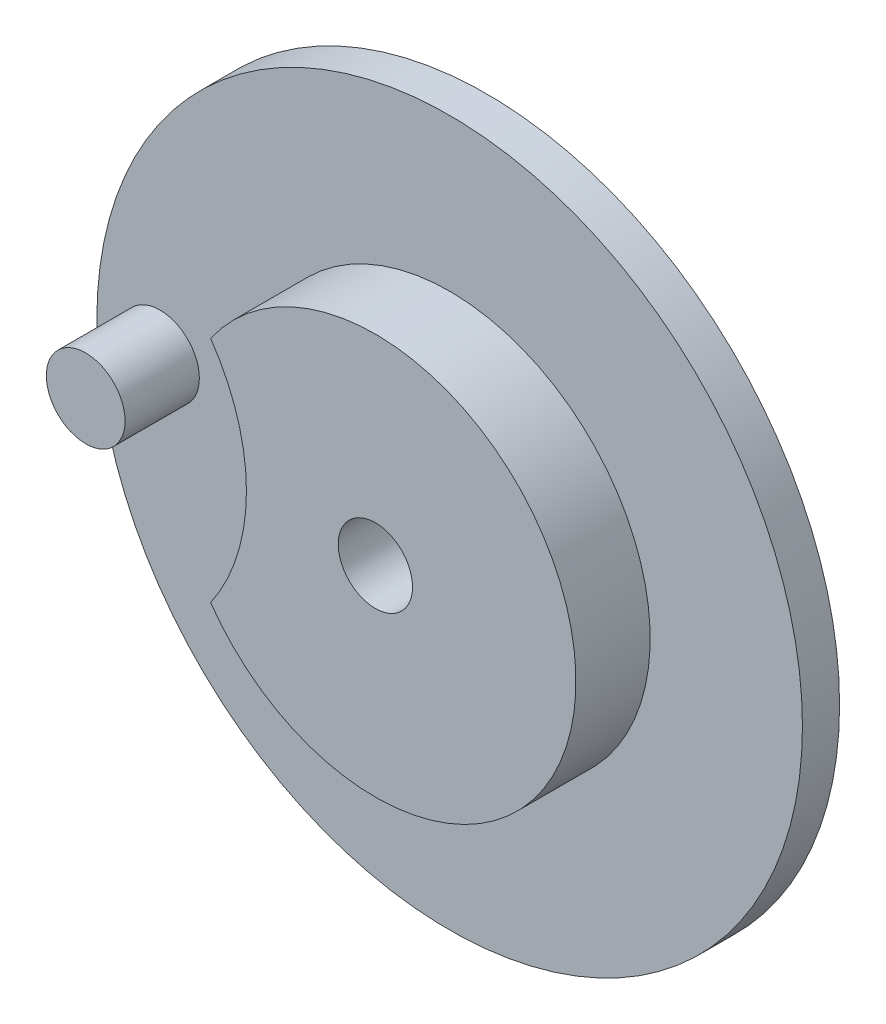
SolidWorks part; units mm, degrees
material "Plain Carbon Steel"
ref_plane "Front Plane" through (0, 0, 0) normal (0, 0, 1) x (1, 0, 0)
ref_plane "Top Plane" through (0, 0, 0) normal (0, 1, 0) x (1, 0, 0)
ref_plane "Right Plane" through (0, 0, 0) normal (1, 0, 0) x (0, 0, -1)
sketch "Disc Profile" plane through (0, 0, 0) normal (0, 0, 1) x (1, 0, 0)
  circle A0 centre (0, 0) radius 47.5
  dimension "D1" = 95
extrude "Disc Ø95x5" add sketch "Disc Profile" along normal blind 5
sketch "Drive Pin Profile" plane through (0, 0, 5) normal (0, 0, 1) x (1, 0, 0)
  circle A0 centre (-39, 0) radius 5.3
  dimension "D2" = 10.6
  dimension "D1" = 39
extrude "Drive Pin Ø10.6" add sketch "Drive Pin Profile" along normal blind 10
sketch "Hub Profile" plane through (0, 0, 5) normal (0, 0, 1) x (1, 0, 0)
  circle A0 centre (0, 0) radius 27
  dimension "D1" = 54
extrude "Hub Ø54x10" add sketch "Hub Profile" along normal blind 10
sketch "Hub Flat Profile" plane through (0, 0, 15) normal (0, 0, 1) x (1, 0, 0)
  circle A0 centre (0, 0) radius 27 construction
  arc A1 (-22.1792, 15.3974) -> (-22.1792, -15.3974) centre (0, 0) ccw
  arc A2 (-22.1792, 15.3974) -> (-22.1792, -15.3974) centre (-44.3585, 0) cw
  circle A3 centre (0, 0) radius 27 construction
  point P2 (-17.3585, 0)
  dimension "D1" = 27
  dimension "D2" = 17.3585
extrude "Hub Flat Cut" cut sketch "Hub Flat Profile" against normal blind 10
sketch "Centre Bore Profile" plane through (0, 0, 15) normal (0, 0, 1) x (1, 0, 0)
  circle A0 centre (0, 0) radius 5
  dimension "D1" = 10
extrude "Centre Bore Ø10" cut sketch "Centre Bore Profile" against normal blind 30
